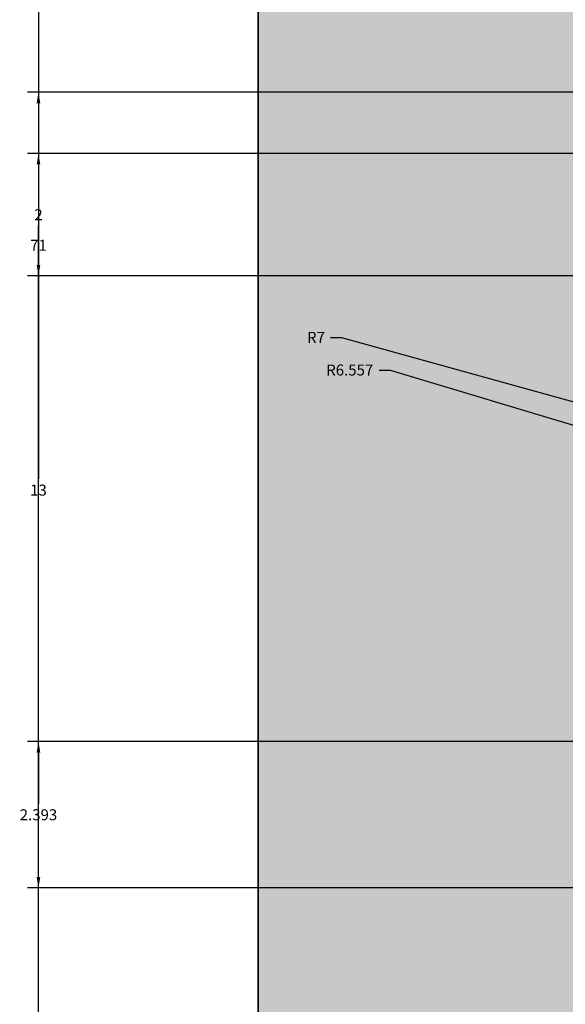
# Model space of a CAD drawing. Units: inches. Extents: x 18 to 59.8, y 2.7 to 81.2.
# Tile 3 of 9: x 18 to 26.9, y 29.5 to 45.6. Entities that reach past the tile are written whole.
import ezdxf

# ---------------------------------------------------------------- set-up
doc = ezdxf.new("R2010")
doc.units = ezdxf.units.IN
doc.header["$MEASUREMENT"] = 0
for name, color, linetype, lineweight in [('A-ANNO-DIMS', 2, 'Continuous', 18), ('A-ELEV', 7, 'Continuous', 35), ('A-ELEV-PATT', 8, 'Continuous', 13)]:
    doc.layers.add(name, color=color, linetype=linetype, lineweight=lineweight)
doc.styles.get("Standard").update_dxf_attribs({"font": 'arial.ttf'})
doc.dimstyles.get("Standard").update_dxf_attribs({"dimtxt": 0.18, "dimasz": 0.18, "dimexe": 0.18, "dimexo": 0.0625, "dimgap": 0.09, "dimtad": 0, "dimtih": 1, "dimtoh": 1, "dimdec": 1, "dimzin": 0, "dimdsep": 46, "dimlunit": 3, "dimtxsty": 'Standard', "dimcen": 0.09, "dimadec": 0, "dimazin": 0, "dimtfac": 1, "dimtdec": 1, "dimtofl": 0, "dimtmove": 0, "dimatfit": 3, "dimfxl": 1, "dimtolj": 1, "dimtzin": 0, "dimarcsym": 0})

# ---------------------------------------------------------------- blocks, each defined once
blk = doc.blocks.new('*D14')
at = {"layer": 'A-ANNO-DIMS', "color": 0, "lineweight": -2, "transparency": 16777216}
for p, q in [((21.797, 77.441), (18.09, 77.441)), ((18.27, 77.261), (18.27, 42.121)), ((18.27, 6.621), (18.27, 41.76)), ((21.797, 6.441), (18.09, 6.441))]:
    blk.add_line(p, q, dxfattribs=at)
at = {"layer": 'A-ANNO-DIMS', "color": 0, "transparency": 16777216}
for points in [[(18.24, 77.261), (18.3, 77.261), (18.27, 77.441)], [(18.24, 6.621), (18.3, 6.621), (18.27, 6.441)]]:
    blk.add_solid(points, dxfattribs=at)
at = {"layer": 'Defpoints', "color": 0, "transparency": 16777216}
for p in [(18.27, 77.441), (21.86, 77.441), (21.86, 6.441)]:
    blk.add_point(p, dxfattribs=at)
at = {"layer": 'A-ANNO-DIMS', "color": 0, "transparency": 16777216, "insert": (18.27, 41.941), "char_height": 0.18, "attachment_point": 5}
blk.add_mtext('\\A1;71', dxfattribs=at)
blk = doc.blocks.new('*D50')
at = {"layer": 'A-ANNO-DIMS', "color": 0, "lineweight": -2, "transparency": 16777216}
for p, q in [((33.949, 44.441), (18.09, 44.441)), ((18.27, 44.261), (18.27, 38.123)), ((18.27, 31.621), (18.27, 37.759)), ((30.344, 31.441), (18.09, 31.441))]:
    blk.add_line(p, q, dxfattribs=at)
at = {"layer": 'A-ANNO-DIMS', "color": 0, "transparency": 16777216}
for points in [[(18.24, 44.261), (18.3, 44.261), (18.27, 44.441)], [(18.24, 31.621), (18.3, 31.621), (18.27, 31.441)]]:
    blk.add_solid(points, dxfattribs=at)
at = {"layer": 'Defpoints', "color": 0, "transparency": 16777216}
for p in [(18.27, 44.441), (34.012, 44.441), (30.406, 31.441)]:
    blk.add_point(p, dxfattribs=at)
at = {"layer": 'A-ANNO-DIMS', "color": 0, "transparency": 16777216, "insert": (18.27, 37.941), "char_height": 0.18, "attachment_point": 5}
blk.add_mtext('\\A1;13', dxfattribs=at)
blk = doc.blocks.new('*D52')
at = {"layer": 'A-ANNO-DIMS', "color": 0, "lineweight": -2, "transparency": 16777216}
for p, q in [((33.949, 43.441), (18.09, 43.441)), ((18.27, 43.261), (18.27, 42.621)), ((18.27, 41.621), (18.27, 42.26)), ((29.286, 41.441), (18.09, 41.441))]:
    blk.add_line(p, q, dxfattribs=at)
at = {"layer": 'A-ANNO-DIMS', "color": 0, "transparency": 16777216}
for points in [[(18.24, 43.261), (18.3, 43.261), (18.27, 43.441)], [(18.24, 41.621), (18.3, 41.621), (18.27, 41.441)]]:
    blk.add_solid(points, dxfattribs=at)
at = {"layer": 'Defpoints', "color": 0, "transparency": 16777216}
for p in [(18.27, 43.441), (34.012, 43.441), (29.348, 41.441)]:
    blk.add_point(p, dxfattribs=at)
at = {"layer": 'A-ANNO-DIMS', "color": 0, "transparency": 16777216, "insert": (18.27, 42.441), "char_height": 0.18, "attachment_point": 5}
blk.add_mtext('\\A1;2', dxfattribs=at)
blk = doc.blocks.new('*D53')
at = {"layer": 'A-ANNO-DIMS', "color": 0, "lineweight": -2, "transparency": 16777216}
for p, q in [((28.196, 33.834), (18.09, 33.834)), ((18.27, 33.654), (18.27, 32.819)), ((18.27, 31.621), (18.27, 32.455)), ((30.344, 31.441), (18.09, 31.441))]:
    blk.add_line(p, q, dxfattribs=at)
at = {"layer": 'A-ANNO-DIMS', "color": 0, "transparency": 16777216}
for points in [[(18.24, 33.654), (18.3, 33.654), (18.27, 33.834)], [(18.24, 31.621), (18.3, 31.621), (18.27, 31.441)]]:
    blk.add_solid(points, dxfattribs=at)
at = {"layer": 'Defpoints', "color": 0, "transparency": 16777216}
for p in [(28.258, 33.834), (18.27, 31.441), (30.406, 31.441)]:
    blk.add_point(p, dxfattribs=at)
at = {"layer": 'A-ANNO-DIMS', "color": 0, "transparency": 16777216, "insert": (18.27, 32.637), "char_height": 0.18, "attachment_point": 5}
blk.add_mtext('\\A1;2.393', dxfattribs=at)
blk = doc.blocks.new('*D69')
at = {"layer": 'A-ANNO-DIMS', "color": 0, "lineweight": -2, "transparency": 16777216}
for p, q in [((23.039, 40.435), (23.219, 40.435)), ((23.219, 40.435), (27.093, 39.36)), ((34.012, 37.351), (34.012, 37.531)), ((33.922, 37.441), (34.102, 37.441))]:
    blk.add_line(p, q, dxfattribs=at)
at = {"layer": 'A-ANNO-DIMS', "color": 0, "transparency": 16777216}
blk.add_solid([(27.101, 39.389), (27.085, 39.331), (27.266, 39.312)], dxfattribs=at)
at = {"layer": 'Defpoints', "color": 0, "transparency": 16777216}
for p in [(27.266, 39.312), (34.012, 37.441)]:
    blk.add_point(p, dxfattribs=at)
at = {"layer": 'A-ANNO-DIMS', "color": 0, "transparency": 16777216, "insert": (22.804, 40.435), "char_height": 0.18, "attachment_point": 5}
blk.add_mtext('\\A1;R7', dxfattribs=at)
blk = doc.blocks.new('*D70')
at = {"layer": 'A-ANNO-DIMS', "color": 0, "lineweight": -2, "transparency": 16777216}
for p, q in [((23.835, 39.903), (24.015, 39.903)), ((24.015, 39.903), (27.611, 38.823)), ((33.973, 36.884), (34.153, 36.884)), ((34.063, 36.794), (34.063, 36.974))]:
    blk.add_line(p, q, dxfattribs=at)
at = {"layer": 'A-ANNO-DIMS', "color": 0, "transparency": 16777216}
blk.add_solid([(27.619, 38.851), (27.602, 38.794), (27.783, 38.771)], dxfattribs=at)
at = {"layer": 'Defpoints', "color": 0, "transparency": 16777216}
for p in [(27.783, 38.771), (34.063, 36.884)]:
    blk.add_point(p, dxfattribs=at)
at = {"layer": 'A-ANNO-DIMS', "color": 0, "transparency": 16777216, "insert": (23.355, 39.903), "char_height": 0.18, "attachment_point": 5}
blk.add_mtext('\\A1;R6.557', dxfattribs=at)

msp = doc.modelspace()

# ---------------------------------------------------------------- hatches: boundary and pattern name
at = {"layer": 'A-ELEV-PATT'}
h = msp.add_hatch(color=256, dxfattribs=at)
h.set_gradient(color1=(255, 255, 255), color2=(199, 200, 202))
h.paths.add_polyline_path([(38.86, 75.4521, 0.4125527), (36.86, 77.4407), (21.86, 77.4407), (21.86, 22.4407), (22.86, 22.4407), (48.86, 22.4407), (48.86, 30.9234, 0.4074473), (48.3302, 31.4407), (30.4061, 31.4407, -0.7603989), (34.0116, 44.4407), (47.86, 44.4407, -0.4142136), (48.86, 43.4407), (48.86, 48.4407, 0.4142136), (47.86, 49.4407), (32.2338, 49.4407, -0.2243142), (27.8411, 52.8427, -0.8480129), (38.86, 61.4407)])
h.paths.add_polyline_path([(55.86, 77.4407), (54.86, 77.4407), (54.86, 22.2407), (55.86, 22.2407)])
h.paths.add_polyline_path([(54.86, 51.5407), (53.4401, 51.5407), (53.4401, 29.6407), (54.86, 29.6407)])
h.paths.add_polyline_path([(54.86, 61.4407), (53.4401, 57.4407), (53.4401, 51.6407), (54.86, 51.6407)])
h.paths.add_polyline_path([(54.86, 29.4407), (54.471, 29.4407), (54.471, 22.2407), (54.86, 22.2407)])
h.paths.add_polyline_path([(55.5745, 22.2407), (54.86, 22.2407), (54.5745, 22.2407), (53.9347, 21.7925), (54.5877, 21.5495)])
h.paths.add_polyline_path([(54.5991, 21.5452), (53.9443, 21.789), (53.9443, 18.4407), (54.5991, 18.4407)])
h.paths.add_polyline_path([(53.9443, 21.789), (53.9347, 21.7925), (53.5816, 21.5452), (53.5816, 18.4407), (53.9443, 18.4407)])
h.paths.add_polyline_path([(53.3648, 20.6928), (52.8956, 21.0646), (52.8956, 18.4407), (53.3648, 18.4407)])
h.paths.add_polyline_path([(52.8956, 21.0646), (50.5775, 19.4407), (50.5775, 18.4407), (52.8956, 18.4407)])
h.paths.add_polyline_path([(53.5816, 21.5452), (52.8956, 21.0646), (53.3648, 20.6928), (53.5816, 20.8447)])
h.paths.add_polyline_path([(26.8109, 19.4407), (24.9672, 20.8407), (24.9672, 18.4407), (26.8109, 18.4407)])
h.paths.add_polyline_path([(24.9672, 20.8407), (24.4165, 20.8427), (24.4165, 18.4407), (24.9672, 18.4407)])
h.paths.add_polyline_path([(24.4165, 20.8427), (24.4165, 21.2589), (24.0588, 21.5305), (24.0301, 21.5183), (24.0301, 18.4407), (24.4165, 18.4407)])
h.paths.add_polyline_path([(24.0301, 21.5183), (23.4165, 21.2589), (23.4165, 18.4407), (24.0301, 18.4407)])
h.paths.add_polyline_path([(24.0301, 21.5183), (24.0588, 21.5305), (23.1234, 22.2407), (22.1234, 22.2407), (23.4165, 21.2589)])
h.paths.add_polyline_path([(24.4165, 21.2589), (24.4165, 20.8427), (24.9672, 20.8407)])
h.paths.add_polyline_path([(47.86, 18.4407), (29.86, 18.4407), (29.86, 6.4407), (30.86, 6.4407), (30.86, 17.4407), (38.86, 17.4407), (46.86, 17.4407), (46.86, 6.4407), (47.86, 6.4407)])
h.paths.add_polyline_path([(54.5756, 15.215), (54.5756, 6.4407), (55.86, 6.4407), (55.86, 18.4407), (47.86, 18.4407), (47.86, 6.4407), (49.1482, 6.4407), (49.1482, 15.215, -1)])
h = msp.add_hatch(dxfattribs=at)
h.set_pattern_fill('ANSI31', color=256, scale=5, angle=45, style=0)
h.paths.add_polyline_path([(54.86, 69.4407), (38.86, 69.4407), (38.86, 61.4407), (54.86, 61.4407)])
h.paths.add_polyline_path([(54.86, 61.4407), (38.86, 61.4407), (36.86, 61.4407, 0.443414), (27.6986, 58.4407), (48.86, 58.4407), (48.86, 57.4407), (53.4401, 57.4407)])
h.paths.add_polyline_path([(37.1661, 59.8577), (37.1187, 59.8577), (37.1187, 59.9399), (37.4994, 59.9399), (37.4994, 59.8577), (37.452, 59.8577, -3.476462)], flags=16)
h.paths.add_polyline_path([(42.66, 59.8391), (42.6125, 59.8391), (42.6125, 59.9213), (42.9933, 59.9213), (42.9933, 59.8391), (42.9458, 59.8391, -3.476462)], flags=16)
h.paths.add_polyline_path([(49.644, 60.0088), (49.5965, 60.0088), (49.5965, 60.091), (49.9773, 60.091), (49.9773, 60.0088), (49.9298, 60.0088, -3.476462)], flags=16)
h.paths.add_polyline_path([(44.4671, 57.0407), (32.6671, 57.0407), (32.6671, 56.0407), (44.4671, 56.0407)])
h.paths.add_polyline_path([(47.86, 43.4407), (46.86, 43.4407), (34.0116, 43.4407, 0.2012983), (29.3481, 41.4407), (47.86, 41.4407, 1)])
h.paths.add_polyline_path([(36.6016, 42.5524), (36.5542, 42.5524), (36.5542, 42.6346), (36.9349, 42.6346), (36.9349, 42.5524), (36.8875, 42.5524, -3.476462)], flags=16)
h.paths.add_polyline_path([(42.9865, 42.578), (42.939, 42.578), (42.939, 42.6603), (43.3198, 42.6603), (43.3198, 42.578), (43.2723, 42.578, -3.476462)], flags=16)
h.paths.add_polyline_path([(54.471, 29.4407), (48.86, 29.4407), (48.86, 22.2407), (54.471, 22.2407)])
h.paths.add_polyline_path([(54.5745, 22.2407), (23.1234, 22.2407), (26.8109, 19.4407), (50.5775, 19.4407)])
h.paths.add_polyline_path([(54.5756, 15.215, 1), (49.1482, 15.215), (49.1482, 6.4407), (54.5756, 6.4407)])
h.paths.add_polyline_path([(49.8323, 9.1225), (49.6657, 9.1225), (49.6657, 12.602), (49.8323, 12.602)], flags=16)
h = msp.add_hatch(color=256, dxfattribs=at)
h.paths.add_polyline_path([(38.86, 17.4407), (30.86, 17.4407), (30.86, 6.4407), (30.96, 6.4407), (30.96, 17.3407), (38.86, 17.3407)])
h.paths.add_polyline_path([(46.86, 17.4407), (38.86, 17.4407), (38.86, 17.3407), (46.76, 17.3407), (46.76, 6.4407), (46.86, 6.4407)])
h.paths.add_polyline_path([(49.8323, 12.602), (49.6657, 12.602), (49.6657, 9.1225), (49.8323, 9.1225)])
h.paths.add_polyline_path([(48.86, 22.4407), (21.86, 22.4407), (21.86, 22.2407), (48.86, 22.2407)])
h.paths.add_polyline_path([(54.86, 29.6407), (48.86, 29.6407), (48.86, 29.4407), (54.86, 29.4407)])
edge = h.paths.add_edge_path()
edge.add_spline(control_points=[(48.3302, 33.5345), (48.1229, 33.671), (47.9155, 33.8074), (47.6839, 33.8336)], knot_values=[0, 0, 0, 0, 0.7121901, 0.7121901, 0.7121901, 0.7121901], degree=3, periodic=0)
edge.add_line((47.6839, 33.8336), (28.2583, 33.8336))
edge.add_arc((34.0631, 36.8836), 6.5573, 207.71831, 208.7099)
edge.add_line((28.3119, 33.7336), (47.6238, 33.7336))
edge.add_spline(control_points=[(47.6238, 33.7336), (47.6461, 33.7341), (47.6685, 33.7345), (47.6905, 33.7336)], knot_values=[0, 0, 0, 0, 0.0667446, 0.0667446, 0.0667446, 0.0667446], degree=3, periodic=0)
edge.add_spline(control_points=[(47.6905, 33.7336), (47.7384, 33.7318), (47.7849, 33.7239), (47.8302, 33.7113)], knot_values=[0.570104, 0.570104, 0.570104, 0.570104, 0.7151116, 0.7151116, 0.7151116, 0.7151116], degree=3, periodic=0)
edge.add_spline(control_points=[(47.8302, 33.7113), (48.0085, 33.6616), (48.1694, 33.5378), (48.3302, 33.4141)], knot_values=[0, 0, 0, 0, 0.570104, 0.570104, 0.570104, 0.570104], degree=3, periodic=0)
edge.add_line((48.3302, 33.4141), (48.3302, 33.5345))

# ---------------------------------------------------------------- linework, layer by layer
at = {"layer": 'A-ELEV'}
msp.add_line((21.86, 22.2407), (21.86, 77.4407), dxfattribs=at)

# ---------------------------------------------------------------- dimensions: what is measured, and where the dimension line sits
at = {"layer": 'A-ANNO-DIMS'}
for base, p1, p2, override, picture, middle in [((18.27, 77.4407), (21.86, 6.4407), (21.86, 77.4407), {"dimdec": 0, "dimlfac": 1, "dimrnd": 0, "dimzin": 0, "dimdsep": 46, "dimlunit": 2}, '*D14', (18.27, 41.9407)), ((18.27, 44.4407), (30.4061, 31.4407), (34.0116, 44.4407), {"dimdec": 0, "dimlfac": 1, "dimrnd": 0, "dimzin": 0, "dimdsep": 46, "dimlunit": 2}, '*D50', (18.27, 37.9407)), ((18.27, 43.4407), (29.3481, 41.4407), (34.0116, 43.4407), {"dimdec": 0, "dimlfac": 1, "dimrnd": 0, "dimzin": 0, "dimdsep": 46, "dimlunit": 2}, '*D52', (18.27, 42.4407)), ((18.27, 31.4407), (28.2583, 33.8336), (30.4061, 31.4407), {"dimdec": 3, "dimlfac": 1, "dimrnd": 0, "dimzin": 0, "dimdsep": 46, "dimlunit": 2}, '*D53', (18.27, 32.6372))]:
    dim = msp.add_linear_dim(base=base, p1=p1, p2=p2, angle=90, dimstyle='Standard', override=override, dxfattribs=at)
    dim.commit()
    dim.dimension.update_dxf_attribs({"geometry": picture, "text_midpoint": middle})
for center, mpoint, override, picture, middle in [((34.0116, 37.4407), (27.2664, 39.3119), {"dimdec": 0, "dimlfac": 1, "dimrnd": 0, "dimzin": 0, "dimdsep": 46, "dimlunit": 2}, '*D69', (22.8041, 40.4346)), ((34.0631, 36.8836), (27.7832, 38.7709), {"dimdec": 3, "dimlfac": 1, "dimrnd": 0, "dimzin": 0, "dimdsep": 46, "dimlunit": 2}, '*D70', (23.3555, 39.9033))]:
    dim = msp.add_radius_dim(center=center, mpoint=mpoint, dimstyle='Standard', override=override, dxfattribs=at)
    dim.commit()
    dim.dimension.update_dxf_attribs({"geometry": picture, "text_midpoint": middle, "dimtype": 164})

doc.saveas('drawing.dxf')
